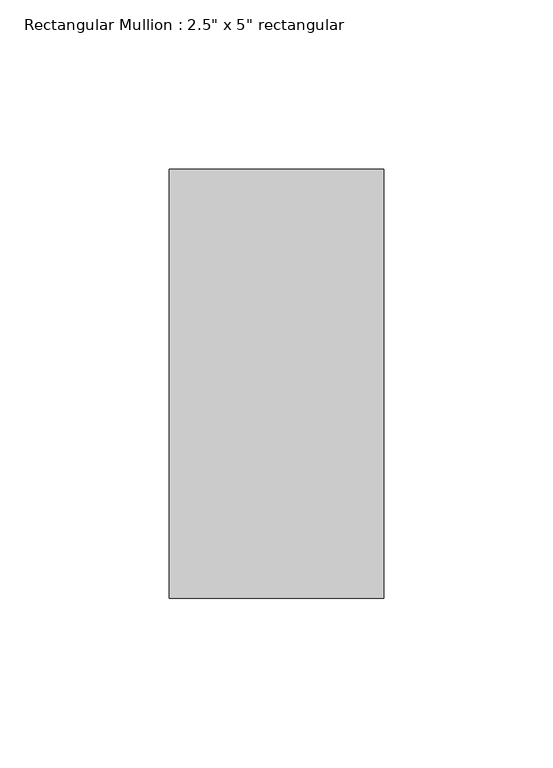
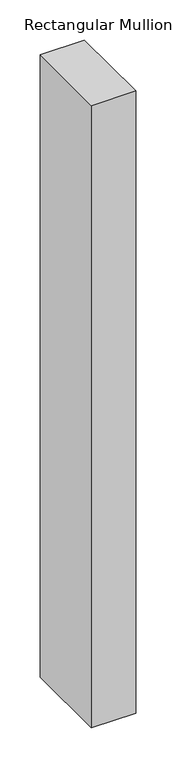
"""IFC4 building model written with IfcOpenShell, lengths in millimetres: member geometry."""

from ifc_helpers import new_model, si_unit, frame, origin, place, context, project, spatial, polyline, outline, extrude, source, transform, mapped, element, save


def member_fc709e3d(model_context):
    return source(origin(), model_context, "Body", "SweptSolid", [
        extrude(outline(polyline([(31.75, 63.5), (31.75, -63.5), (-31.75, -63.5), (-31.75, 63.5), (31.75, 63.5)])), frame((0.0, 0.0, -944.4680153), z_axis=(0.0, 0.0, 1.0), x_axis=(1.0, 0.0, 0.0)), (0.0, 0.0, 1.0), 944.4680153),
    ])


if __name__ == "__main__":
    model = new_model("IFC4")
    model_context = context("Model", 3, world=origin())
    ifc_project = project(units=[si_unit("LENGTHUNIT", "METRE", prefix="MILLI")], contexts=[model_context])
    site = spatial("IfcSite", under=ifc_project)
    building = spatial("IfcBuilding", under=site)
    placement = place(None, origin())
    member_shape = member_fc709e3d(model_context)
    element("IfcMember", 1, ObjectType="Rectangular Mullion : 2.5\" x 5\" rectangular", at=placement, inside=building, context=model_context, shape_type="MappedRepresentation", body=[
        mapped(member_shape, transform((0.0, 0.0, 0.0), x_axis=(1.0, 0.0, 0.0), y_axis=(0.0, 1.0, 0.0), z_axis=(0.0, 0.0, 1.0))),
    ])
    save(model, "model.ifc")

# Revit data of these elements
# Type "Rectangular Mullion : 2.5\" x 5\" rectangular"
#   built-in parameter 1007304 = 0.416667 (stored number, unit not read)
#   built-in parameter 1007301 = 0.104167 (stored number, unit not read)
#   built-in parameter 1007300 = 0.104167 (stored number, unit not read)
# Element 1 (IfcMember, "Rectangular Mullion : 2.5\" x 5\" rectangular")
#   Materials on its faces: "Aluminum"
# Materials
#   "Aluminum": class "Metal", colour RGB 247 247 247, transparency 0, Description = "Aluminum 6061", Cost = 0
